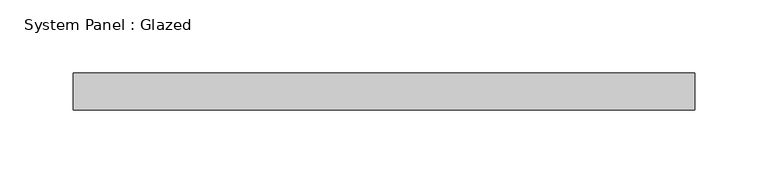
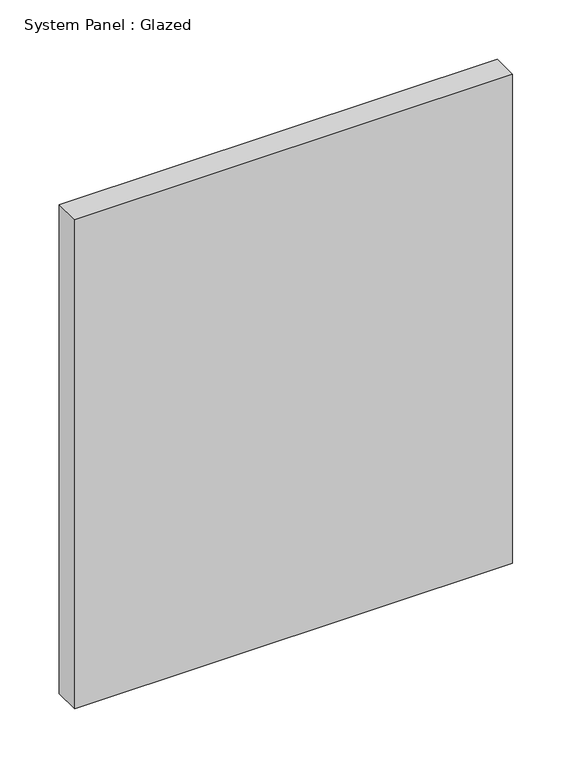
"""IFC4 building model written with IfcOpenShell, lengths in millimetres: plate geometry, System Panel : Glazed."""

from ifc_helpers import new_model, si_unit, origin, origin_with_axes, place, context, project, spatial, polyline, outline, extrude, source, transform, mapped, element, save


def system_panel_glazed_6b1abce8(model_context):
    return source(origin(), model_context, "Body", "SweptSolid", [
        extrude(outline(polyline([(212.725, 19.05), (-212.725, 19.05), (-212.725, 44.45), (212.725, 44.45), (212.725, 19.05)])), origin_with_axes(), (0.0, 0.0, 1.0), 501.65),
    ])


if __name__ == "__main__":
    model = new_model("IFC4")
    model_context = context("Model", 3, world=origin())
    ifc_project = project(units=[si_unit("LENGTHUNIT", "METRE", prefix="MILLI")], contexts=[model_context])
    site = spatial("IfcSite", under=ifc_project)
    building = spatial("IfcBuilding", under=site)
    placement = place(None, origin())
    system_panel_glazed_shape = system_panel_glazed_6b1abce8(model_context)
    element("IfcPlate", 1, ObjectType="System Panel : Glazed", at=placement, inside=building, context=model_context, shape_type="MappedRepresentation", body=[
        mapped(system_panel_glazed_shape, transform((0.0, 0.0, 0.0), x_axis=(1.0, 0.0, 0.0), y_axis=(0.0, 1.0, 0.0), z_axis=(0.0, 0.0, 1.0))),
    ])
    save(model, "model.ifc")

# Revit data of these elements
# Type "System Panel : Glazed"
#   Construction Type Id = "GSP4R"
#   Analytic Construction = "1/8 in Pilkington single glazing"
#   Visual Light Transmittance = 0.9
#   Solar Heat Gain Coefficient = 0.86
#   Heat Transfer Coefficient (U) = 1.18115 BTU/(h·ft²·°F)
#   Define Thermal Properties by = 1
# Element 1 (IfcPlate, "System Panel : Glazed")
#   Materials on its faces: "Glass"
# Materials
#   "Glass": class "Glass", colour RGB 0 128 192, transparency 0.75, Description = "Soda Lime Glass", Cost = 0
